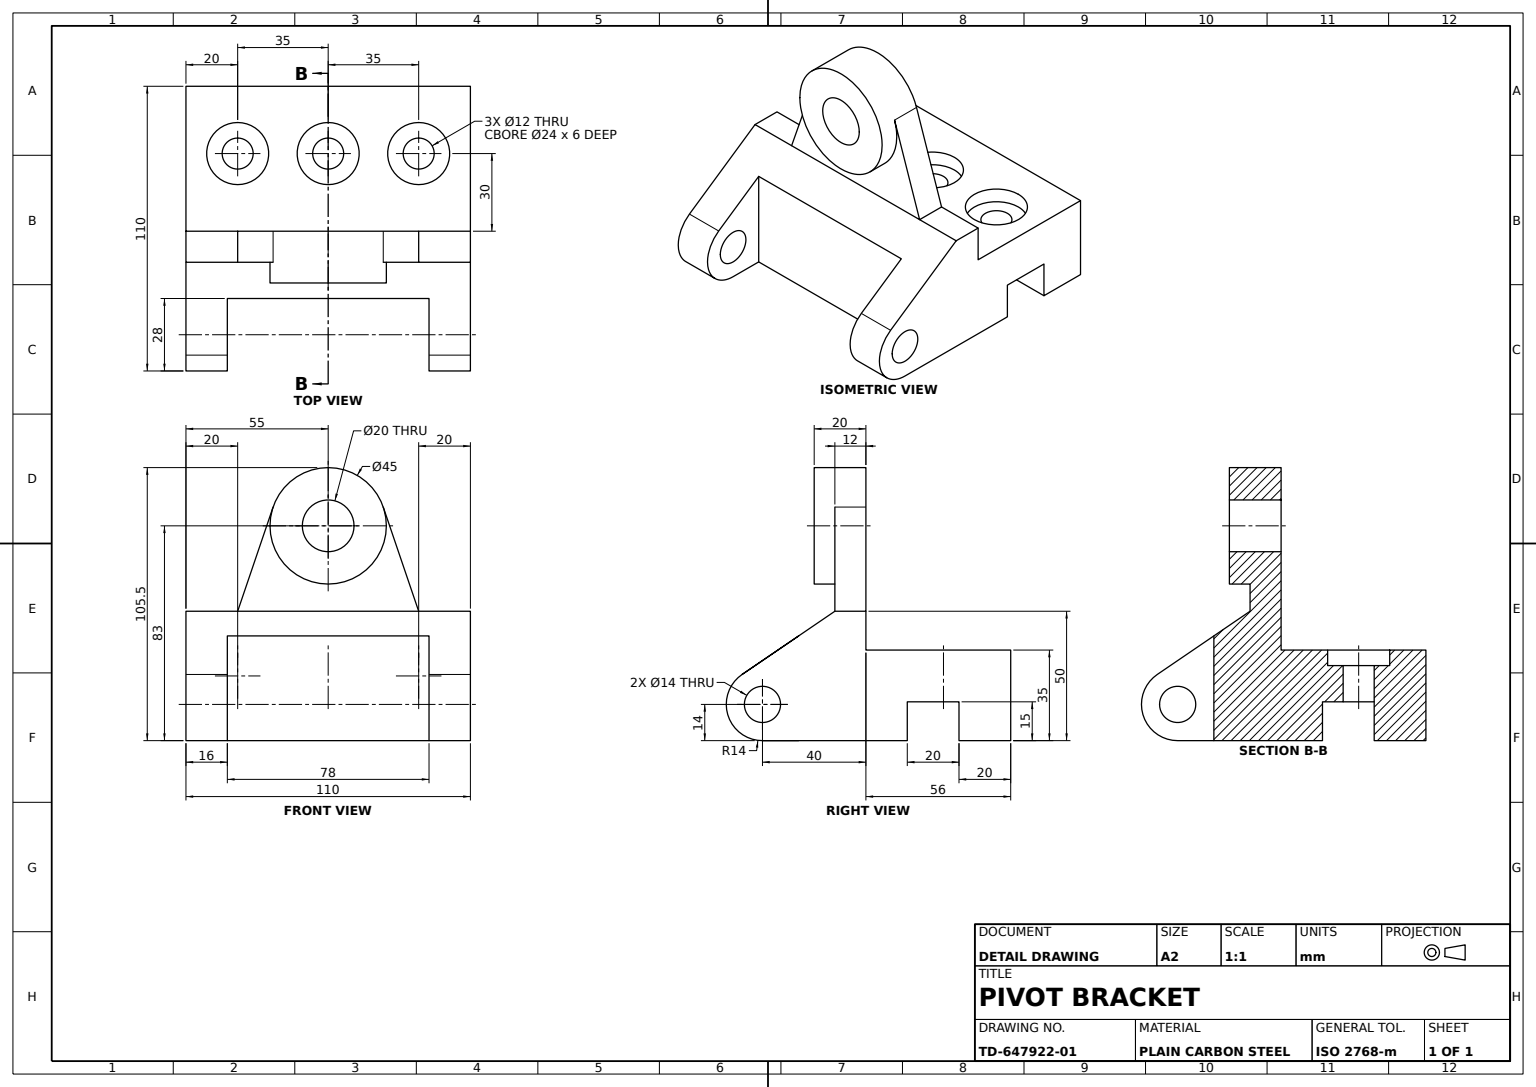
from build123d import *

# Parameters (mm, degrees)
BASE_PROFILE_SKETCH_R             = 7
BASE_BODY_DEPTH                   = 55
RECESS_PROFILE_SKETCH_W           = 28
RECESS_PROFILE_SKETCH_H           = 40.468356276
RECESS_CUT_78_DEPTH               = 39
EYELET_LUG_SKETCH_R               = 22.5
EYELET_LUG_SKETCH_R_2             = 10
EYELET_LUG_20_DEPTH               = 20
EYELET_WEB_12_DEPTH               = 12
COUNTERBORED_HOLES_12_D           = 12
COUNTERBORED_HOLES_12_CBORE_D     = 24
COUNTERBORED_HOLES_12_CBORE_DEPTH = 6


with BuildPart() as part:
    # Base Profile Sketch → Base Body (new, symmetric)
    with BuildSketch(Plane(origin=(0, 0, 0), x_dir=(0, 0, -1), z_dir=(1, 0, 0))):
        with BuildLine():
            Line((40, 0), (20, 0))
            Line((20, 0), (20, 15))
            Line((20, 15), (0, 15))
            Line((0, 15), (0, 0))
            Line((0, 0), (-56, 0))
            ThreePointArc((-56, 0), (-69.379366808, 9.877798669), (-63.878920524, 25.572493741))
            Line((-63.878920524, 25.572493741), (-28, 50))
            Line((-28, 50), (-16, 50))
            Line((-16, 50), (-16, 35))
            Line((-16, 35), (40, 35))
            Line((40, 35), (40, 0))
        make_face()
        with Locations((-56, 14)):
            Circle(BASE_PROFILE_SKETCH_R, mode=Mode.SUBTRACT)
    extrude(amount=BASE_BODY_DEPTH, both=True)

    # Recess Profile Sketch → Recess Cut 78 (cut, symmetric)
    with BuildSketch(Plane(origin=(0, 0, 0), x_dir=(0, 0, -1), z_dir=(1, 0, 0))):
        with Locations((-56, 20.234178138)):
            Rectangle(RECESS_PROFILE_SKETCH_W, RECESS_PROFILE_SKETCH_H)
    extrude(amount=RECESS_CUT_78_DEPTH, both=True, mode=Mode.SUBTRACT)



with BuildPart() as body_2:
    # Eyelet Lug Sketch → Eyelet Lug 20 (new body)
    with BuildSketch(Plane(origin=(0, 0, 16), x_dir=(-1, 0, 0), z_dir=(0, 0, -1))):
        with Locations((0, 83)):
            Circle(EYELET_LUG_SKETCH_R)
        with Locations((0, 83)):
            Circle(EYELET_LUG_SKETCH_R_2, mode=Mode.SUBTRACT)
    extrude(amount=-EYELET_LUG_20_DEPTH)


with BuildPart() as part_1:
    add(part.part)

    add(body_2.part)  # Eyelet Web 12 merges body 2
    # Sketch4_3 → Eyelet Web 12 (add)
    with BuildSketch(Plane(origin=(0, 0, 16), x_dir=(-1, 0, 0), z_dir=(0, 0, -1))):
        with BuildLine():
            Line((-35, 50), (0, 50))
            Line((0, 50), (0, 60.5))
            ThreePointArc((0, 60.5), (-18.294452315, 69.901793463), (-21.299956881, 90.249954267))
            Line((-21.299956881, 90.249954267), (-35, 50))
        make_face()
        with BuildLine():
            Line((0, 60.5), (0, 50))
            Line((0, 50), (35, 50))
            Line((35, 50), (21.299956881, 90.249954267))
            ThreePointArc((21.299956881, 90.249954267), (22.197961954, 86.674300626), (22.5, 83))
            ThreePointArc((22.5, 83), (15.909902577, 67.090097423), (0, 60.5))
        make_face()
    extrude(amount=-EYELET_WEB_12_DEPTH)

    # Counterbored Holes _12 (through all)
    with Locations(Plane(origin=(0, 35, 0), x_dir=(1, 0, 0), z_dir=(0, 1, 0))):
        with Locations((35, 14), (0, 14), (-35, 14)):
            CounterBoreHole(COUNTERBORED_HOLES_12_D / 2, COUNTERBORED_HOLES_12_CBORE_D / 2, COUNTERBORED_HOLES_12_CBORE_DEPTH)


solid = part_1.part
